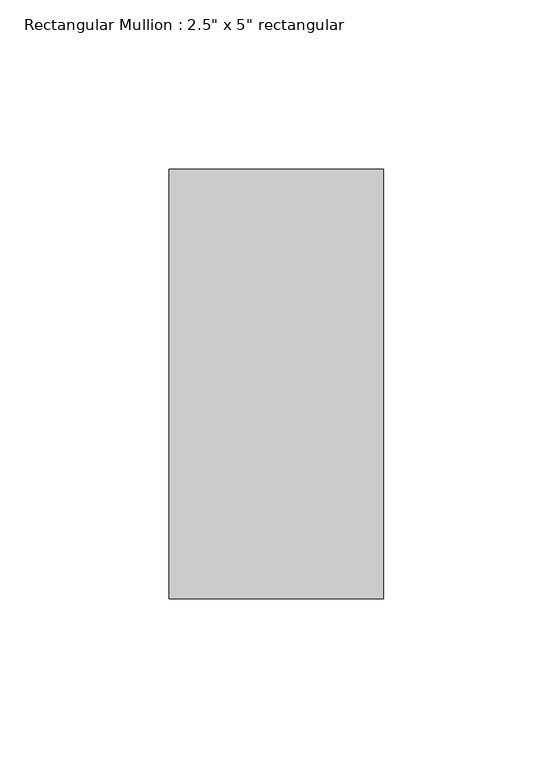
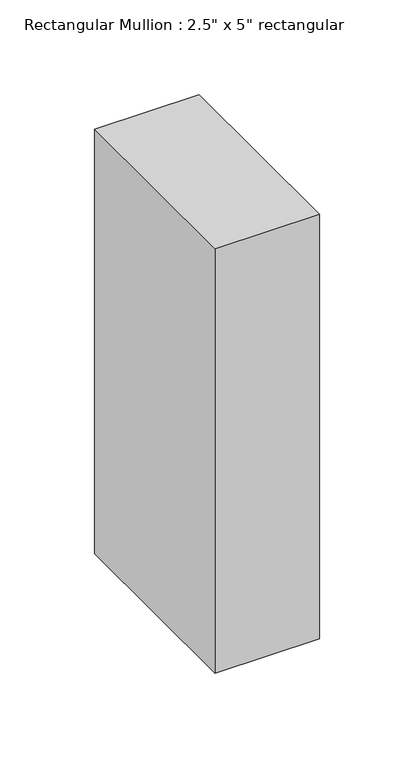
"""IFC4 building model written with IfcOpenShell, lengths in millimetres: member geometry."""

from ifc_helpers import new_model, si_unit, frame, origin, place, context, project, spatial, polyline, outline, extrude, source, transform, mapped, element, save


def member_c327c56d(model_context):
    return source(origin(), model_context, "Body", "SweptSolid", [
        extrude(outline(polyline([(0.0, 63.5), (0.0, -63.5), (-63.5, -63.5), (-63.5, 63.5), (0.0, 63.5)])), frame((0.0, 0.0, -273.05), z_axis=(0.0, 0.0, 1.0), x_axis=(1.0, 0.0, 0.0)), (0.0, 0.0, 1.0), 273.05),
    ])


if __name__ == "__main__":
    model = new_model("IFC4")
    model_context = context("Model", 3, world=origin())
    ifc_project = project(units=[si_unit("LENGTHUNIT", "METRE", prefix="MILLI")], contexts=[model_context])
    site = spatial("IfcSite", under=ifc_project)
    building = spatial("IfcBuilding", under=site)
    placement = place(None, origin())
    member_shape = member_c327c56d(model_context)
    element("IfcMember", 1, ObjectType="Rectangular Mullion : 2.5\" x 5\" rectangular", at=placement, inside=building, context=model_context, shape_type="MappedRepresentation", body=[
        mapped(member_shape, transform((0.0, 0.0, 0.0), x_axis=(1.0, 0.0, 0.0), y_axis=(0.0, 1.0, 0.0), z_axis=(0.0, 0.0, 1.0))),
    ])
    save(model, "model.ifc")

# Revit data of these elements
# Type "Rectangular Mullion : 2.5\" x 5\" rectangular"
#   built-in parameter 1007304 = 0.416667 (stored number, unit not read)
#   built-in parameter 1007301 = 0.104167 (stored number, unit not read)
#   built-in parameter 1007300 = 0.104167 (stored number, unit not read)
# Element 1 (IfcMember, "Rectangular Mullion : 2.5\" x 5\" rectangular")
#   Materials on its faces: "Aluminum"
# Materials
#   "Aluminum": class "Metal", colour RGB 247 247 247, transparency 0, Description = "Aluminum 6061", Cost = 0
